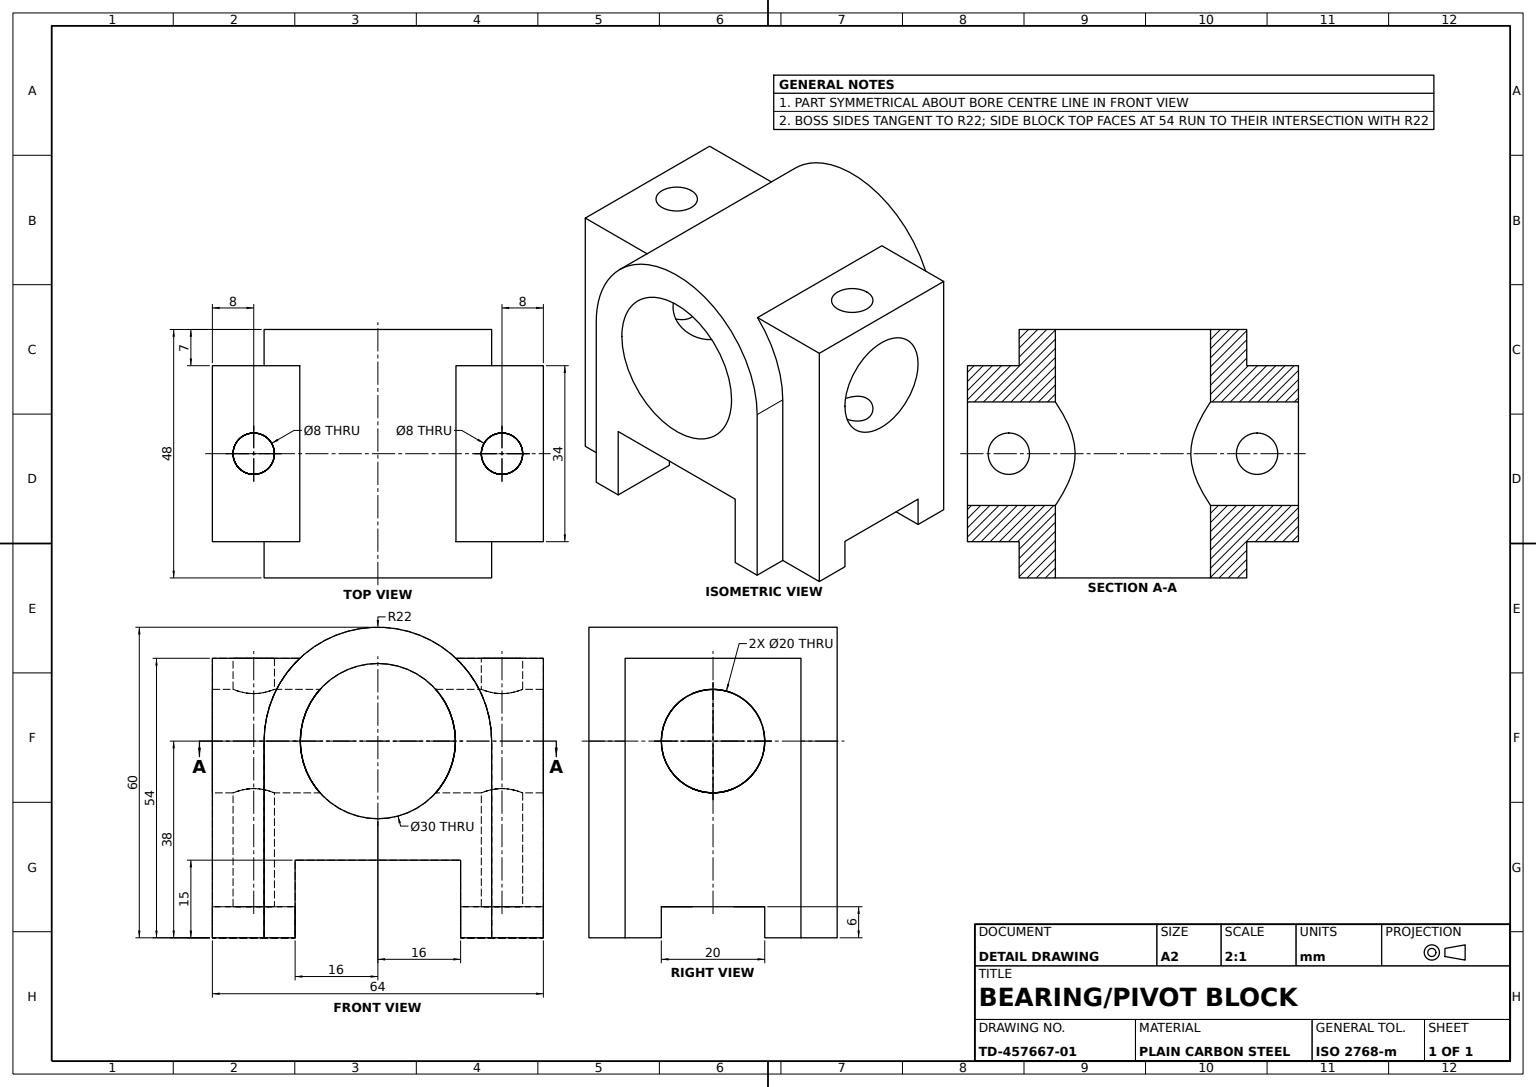
from build123d import *

# Parameters (mm, degrees)
BASE_BLOCK_PROFILE_W       = 64
BASE_BLOCK_PROFILE_H       = 54
BASE_BLOCK_DEPTH           = 17
BEARING_HOUSING_BOSS_DEPTH = 24
MAIN_BORE_PROFILE_R        = 15
MAIN_BORE_PROFILE_W        = 32
MAIN_BORE_PROFILE_H        = 15
MAIN_BORE_DEPTH            = 48
CROSS_HOLES_REACH          = 77.901
CROSS_HOLE_PROFILE_R       = 10
CROSS_HOLE_PROFILE_W       = 20
CROSS_HOLE_PROFILE_H       = 6
TOP_PIN_HOLES_REACH        = 69.201
TOP_PIN_HOLE_PROFILE_R     = 4


with BuildPart() as part:
    # Base Block Profile → Base Block (new, symmetric)
    with BuildSketch(Plane.XY):
        Rectangle(BASE_BLOCK_PROFILE_W, BASE_BLOCK_PROFILE_H)
    extrude(amount=BASE_BLOCK_DEPTH, both=True)

    # Housing Boss Profile → Bearing Housing Boss (add, symmetric)
    with BuildSketch(Plane.XY):
        with BuildLine():
            Line((-22, 11), (-22, -27))
            Line((-22, -27), (22, -27))
            Line((22, -27), (22, 11))
            ThreePointArc((22, 11), (0, 33), (-22, 11))
        make_face()
    extrude(amount=BEARING_HOUSING_BOSS_DEPTH, both=True)

    # Main Bore Profile → Main Bore (cut)
    with BuildSketch(Plane.XY.offset(24)):
        with Locations((0, 11)):
            Circle(MAIN_BORE_PROFILE_R)
        with Locations((0, -19.5)):
            Rectangle(MAIN_BORE_PROFILE_W, MAIN_BORE_PROFILE_H)
    extrude(amount=-MAIN_BORE_DEPTH, mode=Mode.SUBTRACT)

    # Cross Holes: up to this face of the body (flat: up to its plane)
    cross_holes_end = Plane(part.part.faces().sort_by_distance((32, 0, 0))[0])
    # Cross Hole Profile → Cross Holes (cut, up to the picked face)
    with BuildSketch(Plane.ZY.offset(32), mode=Mode.PRIVATE) as cross_holes_sk1:
        with Locations((0, 11)):
            Circle(CROSS_HOLE_PROFILE_R)
    cross_holes_tool1 = split(extrude(cross_holes_sk1.sketch, amount=-CROSS_HOLES_REACH, mode=Mode.PRIVATE), bisect_by=cross_holes_end, keep=Keep.BOTH, mode=Mode.PRIVATE)
    # Cross Hole Profile → Cross Holes (cut, up to the picked face)
    with BuildSketch(Plane.ZY.offset(32), mode=Mode.PRIVATE) as cross_holes_sk2:
        with Locations((0, -24)):
            Rectangle(CROSS_HOLE_PROFILE_W, CROSS_HOLE_PROFILE_H)
    cross_holes_tool2 = split(extrude(cross_holes_sk2.sketch, amount=-CROSS_HOLES_REACH, mode=Mode.PRIVATE), bisect_by=cross_holes_end, keep=Keep.BOTH, mode=Mode.PRIVATE)
    add(cross_holes_tool1.solids().sort_by(Axis((-32, 11, 0), (1, 0, 0)))[0], mode=Mode.SUBTRACT)
    add(cross_holes_tool2.solids().sort_by(Axis((-32, -24, 0), (1, 0, 0)))[0], mode=Mode.SUBTRACT)

    # Top Pin Holes: up to this face of the body (flat: up to its plane)
    top_pin_holes_end = Plane(part.part.faces().sort_by_distance((-24, -21, 0))[0])
    # Top Pin Hole Profile → Top Pin Holes (cut, up to the picked face)
    with BuildSketch(Plane(origin=(0, 27, 0), x_dir=(1, 0, 0), z_dir=(0, 1, 0)), mode=Mode.PRIVATE) as top_pin_holes_sk1:
        with Locations(Location((-24, 0, 0), (0, 0, 270))):
            Circle(TOP_PIN_HOLE_PROFILE_R)
    top_pin_holes_tool1 = split(extrude(top_pin_holes_sk1.sketch, amount=-TOP_PIN_HOLES_REACH, mode=Mode.PRIVATE), bisect_by=top_pin_holes_end, keep=Keep.BOTH, mode=Mode.PRIVATE)
    # Top Pin Hole Profile → Top Pin Holes (cut, up to the picked face)
    with BuildSketch(Plane(origin=(0, 27, 0), x_dir=(1, 0, 0), z_dir=(0, 1, 0)), mode=Mode.PRIVATE) as top_pin_holes_sk2:
        with Locations(Location((24, 0, 0), (0, 0, 270))):
            Circle(TOP_PIN_HOLE_PROFILE_R)
    top_pin_holes_tool2 = split(extrude(top_pin_holes_sk2.sketch, amount=-TOP_PIN_HOLES_REACH, mode=Mode.PRIVATE), bisect_by=top_pin_holes_end, keep=Keep.BOTH, mode=Mode.PRIVATE)
    add(top_pin_holes_tool1.solids().sort_by(Axis((-24, 27, 0), (0, -1, 0)))[0], mode=Mode.SUBTRACT)
    add(top_pin_holes_tool2.solids().sort_by(Axis((24, 27, 0), (0, -1, 0)))[0], mode=Mode.SUBTRACT)


solid = part.part
